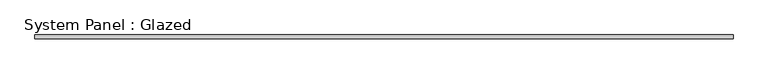
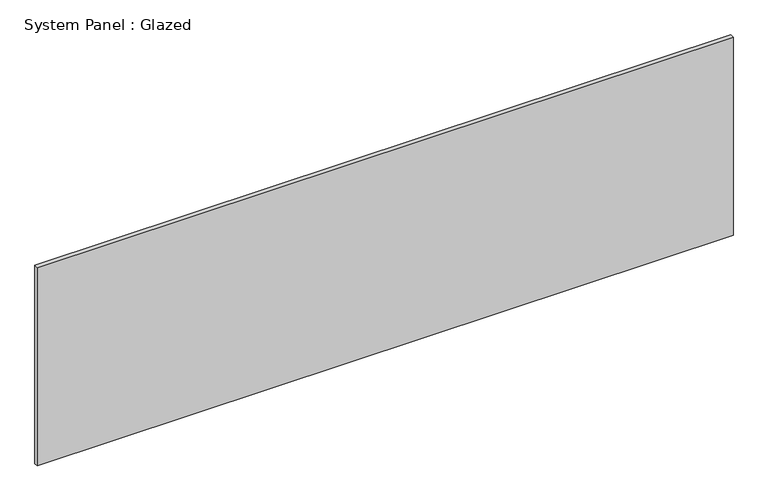
"""IFC4 building model written with IfcOpenShell, lengths in millimetres: plate geometry, System Panel : Glazed."""

from ifc_helpers import new_model, si_unit, origin, origin_with_axes, place, context, project, spatial, polyline, outline, extrude, source, transform, mapped, element, save


def system_panel_glazed_42f91ed4(model_context):
    return source(origin(), model_context, "Body", "SweptSolid", [
        extrude(outline(polyline([(2317.75, 19.05), (-2317.75, 19.05), (-2317.75, 44.45), (2317.75, 44.45), (2317.75, 19.05)])), origin_with_axes(), (0.0, 0.0, 1.0), 1397.0),
    ])


if __name__ == "__main__":
    model = new_model("IFC4")
    model_context = context("Model", 3, world=origin())
    ifc_project = project(units=[si_unit("LENGTHUNIT", "METRE", prefix="MILLI")], contexts=[model_context])
    site = spatial("IfcSite", under=ifc_project)
    building = spatial("IfcBuilding", under=site)
    placement = place(None, origin())
    system_panel_glazed_shape = system_panel_glazed_42f91ed4(model_context)
    element("IfcPlate", 1, ObjectType="System Panel : Glazed", at=placement, inside=building, context=model_context, shape_type="MappedRepresentation", body=[
        mapped(system_panel_glazed_shape, transform((0.0, 0.0, 0.0), x_axis=(1.0, 0.0, 0.0), y_axis=(0.0, 1.0, 0.0), z_axis=(0.0, 0.0, 1.0))),
    ])
    save(model, "model.ifc")

# Revit data of these elements
# Type "System Panel : Glazed"
#   Construction Type Id = "GSP4R"
#   Analytic Construction = "1/8 in Pilkington single glazing"
#   Visual Light Transmittance = 0.9
#   Solar Heat Gain Coefficient = 0.86
#   Heat Transfer Coefficient (U) = 1.18115 BTU/(h·ft²·°F)
# Element 1 (IfcPlate, "System Panel : Glazed")
#   Materials on its faces: "Glass"
# Materials
#   "Glass": class "Glass", colour RGB 0 128 192, transparency 0.75, Description = "Soda Lime Glass", Cost = 0
